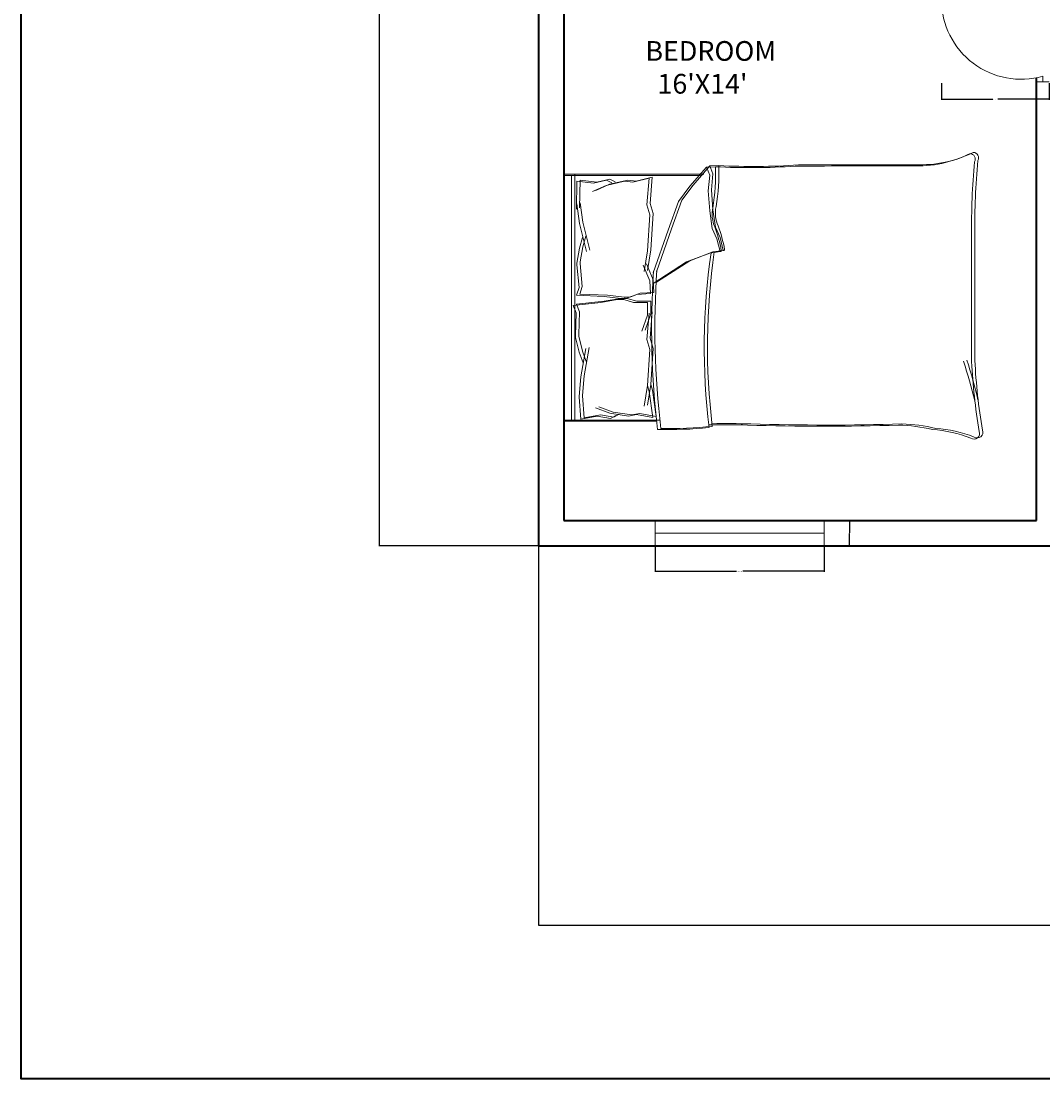
# Model space of a CAD drawing. Units: inches. Extents: x 2185 to 4426, y 1138 to 3073.
# Tile 1 of 14: x 2185 to 2548, y 1138 to 1514. Entities that reach past the tile are written whole.
import ezdxf

# ---------------------------------------------------------------- set-up
doc = ezdxf.new("R2010")
doc.units = ezdxf.units.IN
for name, color, linetype, lineweight in [('A-ANNO-DIMS', 2, 'Continuous', 18), ('A-ANNO-TTLB', 7, 'Continuous', 35), ('A-AREA-IDEN', 7, 'Continuous', 18), ('A-DOOR', 3, 'Continuous', 18), ('A-FURN', 8, 'Continuous', 18), ('A-GLAZ', 4, 'Continuous', 18), ('A-WALL', 7, 'Continuous', 35)]:
    doc.layers.add(name, color=color, linetype=linetype, lineweight=lineweight)
doc.styles.get("Standard").update_dxf_attribs({"font": 'arial.ttf'})
doc.dimstyles.get("Standard").update_dxf_attribs({"dimtxt": 0.18, "dimasz": 0.18, "dimexe": 0.18, "dimexo": 0.0625, "dimgap": 0.09, "dimtad": 0, "dimtih": 1, "dimtoh": 1, "dimdec": 4, "dimzin": 0, "dimdsep": 46, "dimtxsty": 'Standard', "dimcen": 0.09, "dimadec": 0, "dimazin": 0, "dimtfac": 1, "dimtdec": 4, "dimtofl": 0, "dimtmove": 0, "dimatfit": 3, "dimfxl": 1, "dimtolj": 1, "dimtzin": 0, "dimarcsym": 0})

# ---------------------------------------------------------------- blocks, each defined once
blk = doc.blocks.new('BED-DOUBLE')
for p, q in [((0, 93.75), (0, 94.16)), ((0, 94.16), (1.36, 94.16)), ((1.17, 94.16), (49.83, 94.16)), ((3.97, 6.77), (3.97, 94.16)), ((50.74, 96.68), (44.79, 89.9)), ((51.91, 97.09), (45.96, 90.32)), ((53.93, 96.82), (50.74, 96.68, 7.08)), ((51.87, 93.87), (50.74, 96.68)), ((55.1, 97.24), (51.91, 97.09, 7.08)), ((53.04, 94.28), (51.91, 97.09)), ((52.47, 88.62), (53.04, 94.28)), ((0, 93.75), (48.66, 93.75)), ((0, 6.35), (0, 93.75)), ((2.8, 6.35), (2.8, 93.75)), ((4.68, 91.64), (4.5, 81.76)), ((4.68, 91.64), (10.55, 90.94)), ((5.85, 92.05), (5.67, 82.18)), ((5.85, 92.05), (11.72, 91.36)), ((10.55, 90.94), (15.25, 92.03)), ((16.27, 90.59), (11.37, 88.43)), ((11.72, 91.36), (16.42, 92.45)), ((21.63, 91.64), (15.1, 90.17)), ((15.25, 92.03), (17.16, 91.09)), ((22.8, 92.05), (16.27, 90.59)), ((16.42, 92.45), (18.33, 91.51)), ((24.57, 91.29), (21.63, 91.64)), ((25.74, 91.71), (22.8, 92.05)), ((30.31, 92.71), (24.57, 91.29)), ((31.48, 93.13), (25.74, 91.71)), ((29.57, 83.32), (30.31, 92.71)), ((30.74, 83.74), (31.48, 93.13)), ((45.96, 90.32), (42, 84.94)), ((51.3, 88.2), (51.87, 93.87)), ((15.1, 90.17), (10.2, 88.01)), ((44.79, 89.9), (40.83, 84.52)), ((51.87, 81.12), (51.3, 88.2)), ((53.04, 81.54), (52.47, 88.62)), ((4.5, 81.76), (4.65, 83.59)), ((4.65, 83.59), (5.61, 76.65)), ((5.67, 82.18), (5.82, 84.01)), ((5.82, 84.01), (6.78, 77.06)), ((30.59, 79.74), (29.57, 83.32)), ((31.76, 80.16), (30.74, 83.74)), ((40.83, 84.52), (37.15, 74.32)), ((42, 84.94), (38.32, 74.74)), ((29.8, 66.92), (30.59, 79.74)), ((30.97, 67.34), (31.76, 80.16)), ((52.72, 74.89), (51.87, 81.12)), ((53.89, 75.31), (53.04, 81.54)), ((5.61, 76.65), (8.09, 66.74)), ((6.78, 77.06), (9.26, 67.15)), ((55.59, 71.63), (53.89, 75.31)), ((6.72, 71.68), (5.63, 67.91)), ((7.89, 72.1), (6.8, 68.32)), ((37.15, 74.32), (31.79, 59.08)), ((38.32, 74.74), (32.96, 59.49)), ((54.42, 71.21), (52.72, 74.89)), ((56.72, 67.09), (55.59, 71.63)), ((144.91, 27.55), (144.91, 72.56)), ((146.08, 27.96), (146.08, 72.97)), ((5.63, 67.91), (4.64, 62.55)), ((6.8, 68.32), (5.81, 62.97)), ((55.55, 66.68), (54.42, 71.21)), ((28.58, 59.55), (29.8, 66.92)), ((29.75, 59.97), (30.97, 67.34)), ((43.66, 63), (51.87, 66.11)), ((44.83, 63.41), (53.04, 66.53)), ((51.87, 66.11), (55.55, 66.68)), ((53.04, 66.53), (56.72, 67.09)), ((4.64, 62.55), (4.68, 61.96)), ((4.68, 61.96), (5.45, 53.86)), ((5.81, 62.97), (5.85, 62.38)), ((5.85, 62.38), (6.62, 54.28)), ((30.61, 56.23), (28.26, 61.85)), ((31.78, 56.65), (29.43, 62.26)), ((31.79, 55.33), (43.66, 63)), ((32.96, 55.75), (44.83, 63.41)), ((32.06, 52.16), (31.78, 56.65)), ((5.45, 53.86), (4.56, 51.16)), ((6.62, 54.28), (5.73, 51.58)), ((30.89, 51.75), (30.61, 56.23)), ((4.56, 51.16), (14.39, 50.71)), ((4.59, 47.93), (14.37, 48.99)), ((5.73, 51.58), (15.56, 51.13)), ((13.2, 48.57), (19.02, 49.63)), ((14.37, 48.99), (20.19, 50.05)), ((14.39, 50.71), (20.26, 50.02)), ((15.56, 51.13), (21.43, 50.44)), ((19.02, 49.63), (21.4, 49.63)), ((20.19, 50.05), (22.57, 50.05)), ((20.26, 50.02), (22.63, 50.17)), ((21.4, 49.63), (24.84, 48.57)), ((21.43, 50.44), (23.8, 50.59)), ((22.57, 50.05), (26.01, 48.99)), ((22.63, 50.17), (26, 51.44)), ((23.8, 50.59), (27.17, 51.86)), ((26, 51.44), (30.89, 51.75)), ((26.01, 48.99), (30.91, 48.99)), ((27.17, 51.86), (32.06, 52.16)), ((30.91, 48.99), (30.91, 44.49)), ((3.42, 47.51), (13.2, 48.57)), ((4.48, 44.87), (3.42, 47.51)), ((5.65, 45.29), (4.59, 47.93)), ((5.38, 37.16), (5.65, 45.29)), ((24.84, 48.57), (29.74, 48.57)), ((29.74, 48.57), (29.74, 44.08)), ((30.74, 35.86), (31.48, 45.25)), ((4.21, 36.74), (4.48, 44.87)), ((29.74, 44.08), (27.75, 38.33)), ((30.91, 44.49), (28.91, 38.74)), ((29.57, 35.45), (30.31, 44.83)), ((4.21, 36.15), (4.21, 36.74)), ((5.54, 30.86), (4.21, 36.15)), ((5.38, 36.57), (5.38, 37.16)), ((6.7, 31.28), (5.38, 36.57)), ((30.59, 31.86), (29.57, 35.45)), ((31.76, 32.28), (30.74, 35.86)), ((6.86, 27.16), (5.54, 30.86)), ((6.06, 22.14), (7.92, 32.19)), ((8.03, 27.58), (6.7, 31.28)), ((7.23, 22.56), (9.08, 32.6)), ((29.8, 19.04), (30.59, 31.86)), ((30.97, 19.46), (31.76, 32.28)), ((6.7, 15.57), (7.23, 22.56)), ((5.54, 15.15), (6.06, 22.14)), ((28.58, 11.67), (29.8, 19.04)), ((29.75, 12.09), (30.97, 19.46)), ((29.8, 19.04), (30.39, 16.97)), ((30.97, 19.46), (31.56, 17.39)), ((5.5, 14.96), (5.54, 15.15)), ((6.67, 15.37), (6.7, 15.57)), ((7.27, 7.55), (6.67, 15.37)), ((30.39, 16.97), (31.71, 7.65)), ((31.56, 17.39), (32.88, 8.07)), ((6.1, 7.13), (5.5, 14.96)), ((17.55, 9.65), (12.52, 11.5)), ((6.06, 7.12), (11.88, 8.18)), ((7.23, 7.54), (13.05, 8.6)), ((16.38, 9.24), (11.35, 11.09)), ((11.88, 8.18), (16.64, 7.39)), ((13.05, 8.6), (17.81, 7.8)), ((22.99, 8.18), (16.38, 9.24)), ((16.64, 7.39), (18.49, 8.44)), ((24.16, 8.6), (17.55, 9.65)), ((17.81, 7.8), (19.66, 8.86)), ((25.89, 8.71), (22.99, 8.18)), ((27.06, 9.13), (24.16, 8.6)), ((31.71, 7.65), (25.89, 8.71)), ((32.88, 8.07), (27.06, 9.13)), ((1.17, 6.77), (0, 6.77)), ((33.12, 6.35), (0, 6.35)), ((34.29, 6.77), (1.17, 6.77))]:
    blk.add_line(p, q)
for centre, radius, start, end in [((125.57, 139.26), 42.18, 267.4714, 296.4681), ((126.74, 139.68), 42.18, 267.4714, 296.4681), ((144.23, 99.5), 2.02, 332.6588, 86.02), ((145.4, 99.91), 2.02, 332.6588, 86.02), ((388.18, 75.25), 243.28, 174.4998, 180.6351), ((389.35, 75.67), 243.28, 174.4998, 180.6351), ((-12.17, 93.86), 66.17, 349.8763, 2.5657), ((66.41, 333.3), 236.81, 266.9791, 273.8365), ((-11, 94.28), 66.17, 349.8763, 2.5657), ((67.58, 333.72), 236.81, 266.9791, 273.8365), ((124.02, -8244.93), 8342.06, 90.002168, 90.286887), ((125.19, -8244.52), 8342.06, 90.002168, 90.286887), ((64.12, 79.99), 11.38, 168.6608, 203.7384), ((65.29, 80.41), 11.38, 168.6608, 203.7384), ((2.71, 56.97), 54.23, 10.6617, 19.8806), ((3.88, 57.39), 54.23, 10.6617, 19.8806), ((285.85, 32.47), 235.93, 171.7845, 186.9006), ((287.02, 32.89), 235.93, 171.7845, 186.9006), ((55.66, 66.99), 0.337, 250.2464, 1.1377), ((56.83, 67.41), 0.337, 250.2464, 1.1377), ((332.91, 39.06), 301.67, 176.0865, 186.7821), ((334.08, 39.47), 301.67, 176.0865, 186.7821), ((-43.36, -31.49), 194.68, 13.3832, 17.7053), ((-42.19, -31.08), 194.68, 13.3832, 17.7053), ((367.26, 39.18), 222.65, 182.9958, 189.4091), ((368.43, 39.6), 222.65, 182.9958, 189.4091), ((36.75, 155.73), 152.34, 268.7218, 275.604), ((37.92, 156.15), 152.34, 268.7218, 275.604), ((57.01, -305.95), 311.07, 88.4762, 91.0082), ((58.18, -305.53), 311.07, 88.4762, 91.0082), ((92.56, 886.57), 881.98, 268.22771, 271.71854), ((93.72, 886.99), 881.98, 268.22771, 271.71854), ((117.98, -49.19), 54.19, 76.0648, 88.9113), ((119.15, -48.77), 54.19, 76.0648, 88.9113), ((129.68, -39.19), 43.09, 67.9751, 86.652), ((128.51, -39.61), 43.09, 67.9751, 86.652), ((145.78, 1.99), 1.99, 236.1736, 23.4781), ((146.95, 2.41), 1.99, 236.1736, 23.4781)]:
    blk.add_arc(centre, radius, start, end)
blk = doc.blocks.new('DOOR-SGL-36-BED-SW')
for p, q in [((38.25, 31.13), (33.75, 31.13)), ((33.75, 31.13), (36, 31.13)), ((36, 31.13), (36, 29.13)), ((36, 29.13), (0, 29.13)), ((36, 0), (36, 2)), ((33.75, 0), (38.25, 0)), ((38.25, 0), (36, 0))]:
    blk.add_line(p, q)
blk.add_arc((28.22, 29.13), 28.22, 180, 285.9925)
blk = doc.blocks.new('WIN-PLAN-60IN-04')
for p, q in [((0, 9), (0, 0)), ((60, 4.5), (60, 9)), ((60, 9), (60, 0)), ((0, 0), (0, 4.5)), ((0, 4.5), (60, 4.5))]:
    blk.add_line(p, q)
blk = doc.blocks.new('*D80')
at = {"layer": 'A-ANNO-DIMS', "color": 0, "lineweight": -2, "transparency": 16777216}
for p, q in [((2511.77, 1491.8), (2511.77, 1485.95)), ((2550.02, 1491.8), (2550.02, 1485.95)), ((2511.95, 1486.13), (2529.96, 1486.13)), ((2549.84, 1486.13), (2531.83, 1486.13))]:
    blk.add_line(p, q, dxfattribs=at)
at = {"layer": 'A-ANNO-DIMS', "color": 0, "transparency": 16777216}
for points in [[(2511.95, 1486.16), (2511.95, 1486.1), (2511.77, 1486.13)], [(2549.84, 1486.16), (2549.84, 1486.1), (2550.02, 1486.13)]]:
    blk.add_solid(points, dxfattribs=at)
at = {"layer": 'Defpoints', "color": 0, "transparency": 16777216}
for p in [(2511.77, 1491.87), (2550.02, 1491.87), (2550.02, 1486.13)]:
    blk.add_point(p, dxfattribs=at)
at = {"layer": 'A-ANNO-DIMS', "color": 0, "transparency": 16777216, "insert": (2530.89, 1486.13), "char_height": 0.18, "attachment_point": 5}
blk.add_mtext('\\A1;DOOR 38 TYP.', dxfattribs=at)
blk = doc.blocks.new('*D110')
at = {"layer": 'A-ANNO-DIMS', "color": 0, "lineweight": -2, "transparency": 16777216}
for p, q in [((2410.04, 1327.31), (2410.04, 1318.2)), ((2470.04, 1327.31), (2470.04, 1318.2)), ((2410.22, 1318.38), (2438.92, 1318.38)), ((2469.86, 1318.38), (2441.16, 1318.38))]:
    blk.add_line(p, q, dxfattribs=at)
at = {"layer": 'A-ANNO-DIMS', "color": 0, "transparency": 16777216}
for points in [[(2410.22, 1318.41), (2410.22, 1318.35), (2410.04, 1318.38)], [(2469.86, 1318.41), (2469.86, 1318.35), (2470.04, 1318.38)]]:
    blk.add_solid(points, dxfattribs=at)
at = {"layer": 'Defpoints', "color": 0, "transparency": 16777216}
for p in [(2410.04, 1327.38), (2470.04, 1327.38), (2470.04, 1318.38)]:
    blk.add_point(p, dxfattribs=at)
at = {"layer": 'A-ANNO-DIMS', "color": 0, "transparency": 16777216, "insert": (2440.04, 1318.38), "char_height": 0.18, "attachment_point": 5}
blk.add_mtext('\\A1;WINDOW 60 TYP.', dxfattribs=at)
blk = doc.blocks.new('*D111')
at = {"layer": 'A-ANNO-DIMS', "color": 0, "lineweight": -2, "transparency": 16777216}
for p, q in [((2470.1, 1336.38), (2479.22, 1336.38)), ((2479.04, 1336.2), (2479.04, 1332.06)), ((2479.04, 1327.56), (2479.04, 1331.7)), ((2470.1, 1327.38), (2479.22, 1327.38))]:
    blk.add_line(p, q, dxfattribs=at)
at = {"layer": 'A-ANNO-DIMS', "color": 0, "transparency": 16777216}
for points in [[(2479.01, 1336.2), (2479.07, 1336.2), (2479.04, 1336.38)], [(2479.01, 1327.56), (2479.07, 1327.56), (2479.04, 1327.38)]]:
    blk.add_solid(points, dxfattribs=at)
at = {"layer": 'Defpoints', "color": 0, "transparency": 16777216}
for p in [(2470.04, 1336.38), (2479.04, 1336.38), (2470.04, 1327.38)]:
    blk.add_point(p, dxfattribs=at)
at = {"layer": 'A-ANNO-DIMS', "color": 0, "transparency": 16777216, "insert": (2479.04, 1331.88), "char_height": 0.18, "attachment_point": 5}
blk.add_mtext('\\A1;9 TYP.', dxfattribs=at)
blk = doc.blocks.new('*D138')
at = {"layer": 'A-ANNO-DIMS', "color": 0, "lineweight": -2, "transparency": 16777216}
for p, q in [((2368.52, 1327.31), (2368.52, 1192.47)), ((3090.02, 1327.31), (3090.02, 1192.47)), ((2368.7, 1192.65), (2728.88, 1192.65)), ((3089.84, 1192.65), (2729.66, 1192.65))]:
    blk.add_line(p, q, dxfattribs=at)
at = {"layer": 'A-ANNO-DIMS', "color": 0, "transparency": 16777216}
for points in [[(2368.7, 1192.68), (2368.7, 1192.62), (2368.52, 1192.65)], [(3089.84, 1192.68), (3089.84, 1192.62), (3090.02, 1192.65)]]:
    blk.add_solid(points, dxfattribs=at)
at = {"layer": 'Defpoints', "color": 0, "transparency": 16777216}
for p in [(2368.52, 1327.38), (3090.02, 1327.38), (3090.02, 1192.65)]:
    blk.add_point(p, dxfattribs=at)
at = {"layer": 'A-ANNO-DIMS', "color": 0, "transparency": 16777216, "insert": (2729.27, 1192.65), "char_height": 0.18, "attachment_point": 5}
blk.add_mtext('\\A1;721.5', dxfattribs=at)
blk = doc.blocks.new('*D139')
at = {"layer": 'A-ANNO-DIMS', "color": 0, "lineweight": -2, "transparency": 16777216}
for p, q in [((2368.46, 2326.38), (2311.84, 2326.38)), ((2312.02, 2326.2), (2312.02, 1827.06)), ((2312.02, 1327.56), (2312.02, 1826.7)), ((2368.46, 1327.38), (2311.84, 1327.38))]:
    blk.add_line(p, q, dxfattribs=at)
at = {"layer": 'A-ANNO-DIMS', "color": 0, "transparency": 16777216}
for points in [[(2311.99, 2326.2), (2312.05, 2326.2), (2312.02, 2326.38)], [(2311.99, 1327.56), (2312.05, 1327.56), (2312.02, 1327.38)]]:
    blk.add_solid(points, dxfattribs=at)
at = {"layer": 'Defpoints', "color": 0, "transparency": 16777216}
for p in [(2312.02, 2326.38), (2368.52, 2326.38), (2368.52, 1327.38)]:
    blk.add_point(p, dxfattribs=at)
at = {"layer": 'A-ANNO-DIMS', "color": 0, "transparency": 16777216, "insert": (2312.02, 1826.88), "char_height": 0.18, "attachment_point": 5}
blk.add_mtext('\\A1;999', dxfattribs=at)

msp = doc.modelspace()

# ---------------------------------------------------------------- linework, layer by layer
at = {"layer": 'A-ANNO-TTLB'}
msp.add_lwpolyline([(2184.741, 3073.364), (4426.252, 3073.364), (4426.252, 1137.99), (2184.741, 1137.99)], close=True, dxfattribs=at)
at = {"layer": 'A-WALL'}
for p, q in [((2368.519, 2136.303), (2368.519, 1327.377)), ((2368.519, 2136.303), (2368.519, 1327.377)), ((2377.519, 1528.377), (2377.519, 1336.377)), ((2377.519, 1528.377), (2377.519, 1336.377)), ((2545.519, 1336.377), (2545.519, 1493.761)), ((2377.519, 1336.377), (2545.519, 1336.377)), ((2377.519, 1336.377), (2545.519, 1336.377)), ((2368.519, 1327.377), (2635.644, 1327.377))]:
    msp.add_line(p, q, dxfattribs=at)

# ---------------------------------------------------------------- block references
at = {"layer": 'A-DOOR'}
msp.add_blockref('DOOR-SGL-36-BED-SW', (2511.769, 1492.307), dxfattribs=at)
at = {"layer": 'A-FURN'}
msp.add_blockref('BED-DOUBLE', (2377.519, 1365.321), dxfattribs=at)
at = {"layer": 'A-GLAZ'}
msp.add_blockref('WIN-PLAN-60IN-04', (2410.039, 1327.377), dxfattribs=at)

# ---------------------------------------------------------------- texts
at = {"layer": 'A-AREA-IDEN', "insert": (2406.555, 1506.788), "char_height": 7, "attachment_point": 1}
msp.add_mtext_dynamic_manual_height_columns("BEDROOM\\P  16'X14'", width=98.77164, gutter_width=12.5, heights=[0], dxfattribs=at)

# ---------------------------------------------------------------- dimensions: what is measured, and where the dimension line sits
at = {"layer": 'A-ANNO-DIMS'}
dim = msp.add_linear_dim(base=(2312.019, 2326.377), p1=(2368.519, 1327.377), p2=(2368.519, 2326.377), angle=90, dimstyle='Standard', override={"dimdec": 0, "dimlfac": 1, "dimrnd": 0, "dimzin": 0, "dimdsep": 46, "dimlunit": 2}, dxfattribs=at)
dim.commit()
dim.dimension.update_dxf_attribs({"geometry": '*D139', "text_midpoint": (2312.019, 1826.877)})
for base, p1, p2, text, picture, middle in [((2550.019, 1486.128), (2511.769, 1491.866), (2550.019, 1491.866), 'DOOR <> TYP.', '*D80', (2530.894, 1486.128)), ((2470.039, 1318.377), (2410.039, 1327.377), (2470.039, 1327.377), 'WINDOW <> TYP.', '*D110', (2440.039, 1318.377))]:
    dim = msp.add_linear_dim(base=base, p1=p1, p2=p2, text=text, dimstyle='Standard', override={"dimdec": 0, "dimlfac": 1, "dimrnd": 0, "dimzin": 0, "dimdsep": 46, "dimlunit": 2}, dxfattribs=at)
    dim.commit()
    dim.dimension.update_dxf_attribs({"geometry": picture, "text_midpoint": middle})
dim = msp.add_linear_dim(base=(2479.039, 1336.377), p1=(2470.039, 1327.377), p2=(2470.039, 1336.377), angle=90, text='<> TYP.', dimstyle='Standard', override={"dimdec": 0, "dimlfac": 1, "dimrnd": 0, "dimzin": 0, "dimdsep": 46, "dimlunit": 2}, dxfattribs=at)
dim.commit()
dim.dimension.update_dxf_attribs({"geometry": '*D111', "text_midpoint": (2479.039, 1331.877)})
dim = msp.add_linear_dim(base=(3090.019, 1192.648), p1=(2368.519, 1327.377), p2=(3090.019, 1327.377), dimstyle='Standard', override={"dimdec": 1, "dimlfac": 1, "dimrnd": 0, "dimzin": 0, "dimdsep": 46, "dimlunit": 2}, dxfattribs=at)
dim.commit()
dim.dimension.update_dxf_attribs({"geometry": '*D138', "text_midpoint": (2729.269, 1192.648)})

doc.saveas('drawing.dxf')
